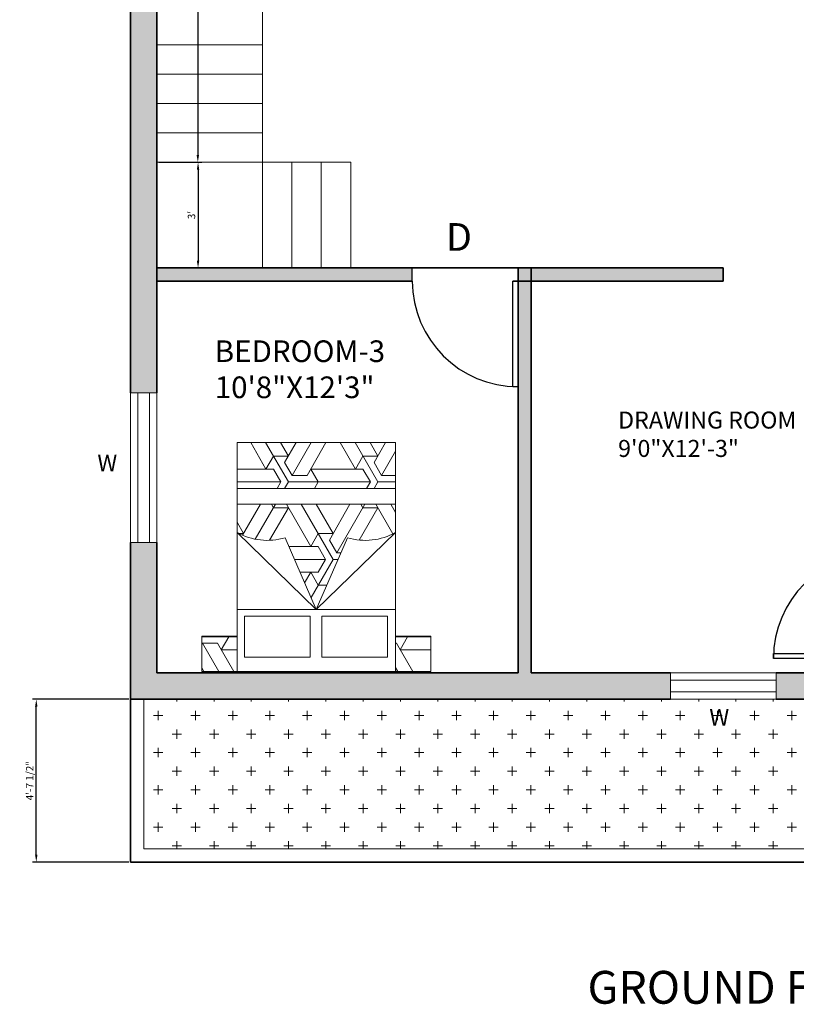
# Model space of a CAD drawing. Units: inches. Extents: x 1878 to 2382, y 1889 to 2524.
# Tile 1 of 2: x 1878 to 2143, y 1889 to 2225. Entities that reach past the tile are written whole.
import ezdxf

# ---------------------------------------------------------------- set-up
doc = ezdxf.new("R2010")
doc.units = ezdxf.units.IN
for name, color, linetype, lineweight in [('A-ANNO-DIMS', 2, 'Continuous', 18), ('A-ANNO-TEXT', 7, 'Continuous', 18), ('A-ANNO-TITL', 7, 'Continuous', 30), ('A-AREA-IDEN', 7, 'Continuous', 18), ('A-DOOR', 4, 'Continuous', 25), ('A-FLOR-STRS', 7, 'Continuous', 18), ('A-FURN', 8, 'Continuous', 18), ('A-FURN-PATT', 252, 'Continuous', 13), ('A-WALL', 7, 'Continuous', 35), ('A-WALL-PATT', 251, 'Continuous', 13), ('L-PLNT', 3, 'Continuous', 18), ('L-PLNT-PATT', 3, 'Continuous', 13), ('windows', 5, 'Continuous', 18)]:
    doc.layers.add(name, color=color, linetype=linetype, lineweight=lineweight)
doc.styles.get("Standard").update_dxf_attribs({"font": 'arial.ttf'})
doc.dimstyles.new('ISO-25', dxfattribs={"dimtxt": 2.5, "dimasz": 2.5, "dimexe": 1.25, "dimexo": 0.625, "dimtad": 1, "dimlunit": 3, "dimtxsty": 'Standard', "dimcen": 2.5, "dimadec": 0, "dimazin": 0, "dimtfac": 1, "dimtmove": 0, "dimatfit": 3, "dimfxl": 1, "dimarcsym": 0})

# ---------------------------------------------------------------- blocks, each defined once
blk = doc.blocks.new('*D9')
at = {"layer": 'A-ANNO-DIMS', "color": 0, "lineweight": -2, "transparency": 16777216}
for p, q in [((1925.866440692248, 2286.068149098085), (1940.420566168725, 2286.068149098085)), ((1939.170566168725, 2283.568149098085), (1939.170566168725, 2178.568149098085)), ((1925.866440692248, 2176.068149098085), (1940.420566168725, 2176.068149098085))]:
    blk.add_line(p, q, dxfattribs=at)
at = {"layer": 'A-ANNO-DIMS', "color": 0, "transparency": 16777216}
for points in [[(1938.753899502058, 2283.568149098085), (1939.587232835391, 2283.568149098085), (1939.170566168725, 2286.068149098085)], [(1938.753899502058, 2178.568149098085), (1939.587232835391, 2178.568149098085), (1939.170566168725, 2176.068149098085)]]:
    blk.add_solid(points, dxfattribs=at)
at = {"layer": 'Defpoints', "color": 0, "transparency": 16777216}
for p in [(1925.241440692248, 2286.068149098085), (1925.241440692248, 2176.068149098085), (1939.170566168725, 2176.068149098085)]:
    blk.add_point(p, dxfattribs=at)
at = {"layer": 'A-ANNO-DIMS', "color": 0, "transparency": 16777216, "insert": (1937.269133699421, 2231.068149098084), "char_height": 2.5, "attachment_point": 5, "rotation": 90}
blk.add_mtext('9\'-2"', dxfattribs=at)
blk = doc.blocks.new('*D11')
at = {"layer": 'A-ANNO-DIMS', "color": 0, "lineweight": -2, "transparency": 16777216}
for p, q in [((1925.866440692248, 2176.068149098085), (1940.498560281259, 2176.068149098085)), ((1939.248560281259, 2173.568149098085), (1939.248560281259, 2142.568149098085)), ((1925.866440692248, 2140.068149098085), (1940.498560281259, 2140.068149098085))]:
    blk.add_line(p, q, dxfattribs=at)
at = {"layer": 'A-ANNO-DIMS', "color": 0, "transparency": 16777216}
for points in [[(1938.831893614593, 2173.568149098085), (1939.665226947926, 2173.568149098085), (1939.248560281259, 2176.068149098085)], [(1938.831893614593, 2142.568149098085), (1939.665226947926, 2142.568149098085), (1939.248560281259, 2140.068149098085)]]:
    blk.add_solid(points, dxfattribs=at)
at = {"layer": 'Defpoints', "color": 0, "transparency": 16777216}
for p in [(1925.241440692248, 2176.068149098085), (1925.241440692248, 2140.068149098085), (1939.248560281259, 2140.068149098085)]:
    blk.add_point(p, dxfattribs=at)
at = {"layer": 'A-ANNO-DIMS', "color": 0, "transparency": 16777216, "insert": (1937.346275151655, 2158.068149098085), "char_height": 2.5, "attachment_point": 5, "rotation": 90}
blk.add_mtext("3'", dxfattribs=at)
blk = doc.blocks.new('*U12')
for p, q in [((-36, 4e-16), (-36, 4)), ((0, 0), (0, 3.999999999999999))]:
    blk.add_line(p, q)
blk.add_lwpolyline([(0, 0), (-7.1e-15, -36), (-1.750000000000007, -36), (-1.75, 4e-16)], close=True)
blk.add_arc((0, 0), 36, 180, 270)
blk = doc.blocks.new('*U2')
for p, q in [((0, 0), (-1e-16, -3.999999999999999)), ((36, -4e-16), (36, -3.999999999999999))]:
    blk.add_line(p, q)
blk.add_lwpolyline([(0, 0), (5.2e-15, 36), (1.750000000000006, 36), (1.749999999999998, -7e-16)], close=True)
blk.add_arc((0, 0), 36, 0, 90)
blk = doc.blocks.new('BED-DOUBLE-WITH-NIGHTSTANDS')
for p, q in [((39.00041612759128, 21.08000700798311), (12.00041612759128, 47.34561457886321)), ((39.00041612759128, 21.08000700798311), (66.00041612759127, 47.34561457886321)), ((39.00041612759128, 21.08000700798311), (28.35091833014235, 45.54110342781223)), ((39.00041612759128, 21.08000700798311), (49.64991392504021, 45.54110342781223)), ((66.00041612759127, 21.08000700798311), (12.00041612759128, 21.08000700798311)), ((36.91574546573361, 4.839445541926579), (36.91574546573361, 18.8744984206578)), ((40.91574546573361, 4.839445541926579), (40.91574546573361, 18.8744984206578)), ((0.0004161275912793, 0.0002775178572847), (0.0004161275912793, 12.00027751785728)), ((0.0004161275912793, 12.00027751785728), (12.00041612759128, 12.00027751785728)), ((78.00041612759128, 12.00027751785728), (66.00041612759127, 12.00027751785728)), ((78.00041612759128, 12.00027751785728), (78.00041612759128, 0.0002775178572847)), ((12.00041612759128, 0.0002775178572847), (0.0004161275912793, 0.0002775178572847)), ((66.00041612759127, 0.0002775178572847), (78.00041612759128, 0.0002775178572847))]:
    blk.add_line(p, q)
for points in [[(66.00041612759127, 78.00027751785728), (12.00041612759128, 78.00027751785728), (12.00041612759128, 0.0002775178572847), (66.00041612759127, 0.0002775178572847)], [(66.00041612759127, 56.96965028294471), (12.00041612759128, 56.96965028294471), (12.00041612759128, 62.38317077163083), (66.00041612759127, 62.38317077163083)]]:
    blk.add_lwpolyline(points, close=True)
for points in [[(36.91574546573361, 4.839445541926579), (14.53815381501522, 4.839445541926579), (14.53815381501522, 18.8744984206578), (36.91574546573361, 18.8744984206578)], [(40.91574546573361, 18.8744984206578), (63.29333711645199, 18.8744984206578), (63.29333711645199, 4.839445541926579), (40.91574546573361, 4.839445541926579)]]:
    blk.add_lwpolyline(points)
for centre, start, end in [((22.35293988504668, 66.17141739726458), 241.1931034301566, 286.2110586149389), ((55.64789237013588, 66.17141739726458), 253.7889413850611, 298.8068965698434)]:
    blk.add_arc(centre, 21.48454327897181, start, end)
blk = doc.blocks.new('WIN-51IN')
for p, q in [((4.500440692245319, 51.00020935019097), (0.0004406922455473, 51.00020935019074)), ((0.0004406922455473, 51.00020935019074), (9.000440692245093, 51.00020935019142)), ((0.0004406922482758, 0.0002093501907439), (0.0004406922441831, 51.00020935019074)), ((2.500440692248048, 0.0002093501907439), (2.500440692245319, 51.00020935019097)), ((6.500440692248048, 0.0002093501911986), (6.500440692245319, 51.0002093501912)), ((9.000440692245318, 51.0002093501912), (9.000440692247594, 0.0002093501911986)), ((0.0004406922482758, 0.0002093501907439), (9.000440692247821, 0.0002093501911986)), ((9.000440692247821, 0.0002093501911986), (4.500440692248048, 0.0002093501911986))]:
    blk.add_line(p, q)
blk = doc.blocks.new('*D27')
at = {"layer": 'A-ANNO-DIMS', "color": 0, "lineweight": -2, "transparency": 16777216}
for p, q in [((1915.616441000001, 1993.068149000001), (1882.891441000001, 1993.068149000001)), ((1884.141441000002, 1940.068149000001), (1884.141441000002, 1990.568149000001)), ((1915.616441000001, 1937.568149000001), (1882.891441000001, 1937.568149000001))]:
    blk.add_line(p, q, dxfattribs=at)
at = {"layer": 'A-ANNO-DIMS', "color": 0, "transparency": 16777216}
for points in [[(1883.724774333335, 1990.568149000001), (1884.558107666668, 1990.568149000001), (1884.141441000002, 1993.068149000001)], [(1883.724774333335, 1940.068149000001), (1884.558107666668, 1940.068149000001), (1884.141441000002, 1937.568149000001)]]:
    blk.add_solid(points, dxfattribs=at)
at = {"layer": 'Defpoints', "color": 0, "transparency": 16777216}
for p in [(1884.141441000002, 1993.068149000001), (1916.241441000001, 1993.068149000001), (1916.241441000001, 1937.568149000001)]:
    blk.add_point(p, dxfattribs=at)
at = {"layer": 'A-ANNO-DIMS', "color": 0, "transparency": 16777216, "insert": (1882.223807984995, 1965.318148999999), "char_height": 2.5, "attachment_point": 5, "rotation": 90}
blk.add_mtext('4\'-7 1/2"', dxfattribs=at)

msp = doc.modelspace()

# ---------------------------------------------------------------- hatches: boundary and pattern name
at = {"layer": 'A-FURN-PATT'}
h = msp.add_hatch(dxfattribs=at)
h.set_pattern_fill('ESCHER', color=256, angle=180)
h.set_pattern_definition([(240, (4377.911806630984, 4495.575865926148), (30.47999998809242, 6.8748365e-09), [27.94, -2.539999999999999]), (360, (4377.911806630984, 4495.575865926148), (-15.23999999999999, 26.39645429360001), [27.94, -2.54]), (120, (4377.911806630984, 4495.575865926148), (-30.47999998809242, 6.874844e-09), [27.94, -2.539999999999999]), (240, (4375.371806630983, 4495.575865926148), (30.47999998809242, 6.8748365e-09), [5.079999999999999, -25.4]), (120, (4375.371806630983, 4495.575865926148), (-30.47999998809242, 6.874844e-09), [5.079999999999999, -25.4]), (240, (4379.181806630984, 4493.376161410148), (30.47999998809242, 6.8748365e-09), [5.079999999999999, -25.4]), (360, (4379.181806630984, 4493.376161410148), (-15.23999999999999, 26.39645429360001), [5.08, -25.4]), (120, (4379.181806630984, 4497.775570442148), (-30.47999998809242, 6.874844e-09), [5.079999999999999, -25.4]), (360, (4379.181806630984, 4497.775570442148), (-15.23999999999999, 26.39645429360001), [5.08, -25.4]), (240, (4388.071806630984, 4495.575865926148), (30.47999998809242, 6.8748365e-09), [5.079999999999999, -25.4]), (120, (4388.071806630984, 4495.575865926148), (-30.47999998809242, 6.874844e-09), [5.079999999999999, -25.4]), (240, (4372.831806630983, 4504.374684015548), (30.47999998809242, 6.8748365e-09), [5.079999999999999, -25.4]), (360, (4372.831806630983, 4504.374684015548), (-15.23999999999999, 26.39645429360001), [5.08, -25.4]), (120, (4372.831806630983, 4486.777047836748), (-30.47999998809242, 6.874844e-09), [5.079999999999999, -25.4]), (360, (4372.831806630983, 4486.777047836748), (-15.23999999999999, 26.39645429360001), [5.08, -25.4]), (180, (4372.831806630983, 4491.176456868749), (15.24, -26.39645429360001), [17.78, -12.7]), (180, (4372.831806630983, 4499.975274983547), (15.24, -26.39645429360001), [17.78, -12.7]), (300, (4376.641806630983, 4488.976752352748), (30.47999998809242, -6.8748546e-09), [17.78, -12.7]), (300, (4384.261806630984, 4493.376161410148), (30.47999998809242, -6.8748546e-09), [17.78, -12.7]), (59.99999999999997, (4384.261806630984, 4497.775570442148), (-15.2399999880924, 26.39645430047486), [17.78, -12.7]), (59.99999999999997, (4376.641806630983, 4502.174979499549), (-15.2399999880924, 26.39645430047486), [17.78, -12.7])])
h.paths.add_polyline_path([(1979.526416127591, 2023.596007007983), (1990.17591392504, 2048.057103427812, 0.1989938127017903), (2006.526416127591, 2049.861614578864), (2006.526416127591, 2059.485650282945), (1952.526416127591, 2059.485650282945), (1952.526416127591, 2049.861614578863, 0.1989938127017848), (1968.876918330142, 2048.057103427812)])
h.paths.add_polyline_path([(1952.526416127591, 2064.899170771631), (2006.526416127591, 2064.899170771631), (2006.526416127591, 2080.516277517857), (1952.526416127591, 2080.516277517857)])
h.paths.add_polyline_path([(1940.526416127591, 2002.516277517857), (1952.526416127591, 2002.516277517857), (1952.526416127591, 2014.516277517858), (1940.526416127591, 2014.516277517858)])
h.paths.add_polyline_path([(2006.526416127591, 2002.516277517857), (2018.526416127591, 2002.516277517857), (2018.526416127591, 2014.516277517858), (2006.526416127591, 2014.516277517858)])
at = {"layer": 'A-WALL-PATT'}
h = msp.add_hatch(color=256, dxfattribs=at)
h.dxf.hatch_style = 1
h.paths.add_polyline_path([(1925.241440692247, 2376.261341107433), (1916.241440692247, 2376.261341107433), (1916.241440692247, 2322.068149098084), (1920.741440692247, 2322.068149098084), (1925.241440692247, 2322.068149098084)])
h.paths.add_polyline_path([(1925.241440692247, 2286.140121582637), (1916.241440692247, 2286.068149098084), (1916.241440692247, 2097.50720935019), (1920.741440692247, 2097.50720935019), (1925.241440692246, 2097.50720935019)])
h.paths.add_polyline_path([(1925.241440692246, 2046.50720935019), (1916.241440692247, 2046.50720935019), (1916.241440692247, 1993.068149098084), (1925.241440692247, 1993.068149098084), (2100.228537208572, 1993.068149098084), (2100.228537208572, 1997.568149098084), (2100.228537208572, 2002.068149098084), (2052.741440692247, 2002.068149098084), (2052.741440692247, 2135.568149098084), (2048.241440692248, 2135.568149098084), (2048.241440692248, 2002.068149098084), (1925.241440692246, 2002.068149098084)])
h.paths.add_polyline_path([(2175.741440692247, 2006.934770096195), (2175.253494205439, 2006.934770096195), (2171.241440692247, 2006.934770096195), (2171.241440692247, 2002.068149098084), (2136.228537208572, 2002.068149098084), (2136.228537208572, 1993.068149098084), (2171.241440692247, 1993.068149098084), (2175.741440692247, 1993.068149098084)])
h.paths.add_polyline_path([(1925.241440692247, 2492.568149098084), (2018.709393843749, 2492.568149098085), (2018.709393843749, 2497.068149098084), (2018.709393843749, 2501.568149098084), (1916.241440692247, 2501.568149098084), (1916.241440692247, 2427.261341107433), (1925.241440692247, 2427.261341107433)])
h.paths.add_polyline_path([(2324.241440692247, 2501.568149098084), (2052.741440692247, 2501.568149098084), (2052.741440692247, 2497.068149098084), (2319.741440692247, 2497.068149098084), (2319.741440692247, 2446.568149098084), (2324.241440692247, 2446.568149098084)])
h.paths.add_polyline_path([(2110.637963685758, 2446.568149098085), (2052.741440692248, 2446.568149098085), (2052.741440692247, 2492.568149098085), (2048.241440692248, 2492.568149098085), (2048.241440692248, 2446.568149098084), (1976.241440692247, 2446.568149098084), (1976.241440692247, 2442.068149098084), (2048.241440692248, 2442.068149098084), (2048.241440692248, 2326.568149098084), (2052.741440692248, 2326.568149098084), (2052.741440692248, 2442.068149098085), (2110.637963685758, 2442.068149098085), (2110.637963685758, 2444.318149098084)])
h.paths.add_polyline_path([(2100.741440692248, 2326.568149098084), (2052.741440692248, 2326.568149098084), (2052.741440692248, 2322.068149098084), (2100.741440692248, 2322.068149098084)])
h.paths.add_polyline_path([(2052.741440692248, 2326.568149098084), (2048.241440692248, 2326.568149098084), (2048.241440692248, 2322.068149098084), (2052.741440692248, 2322.068149098084)])
h.paths.add_polyline_path([(2048.241440692248, 2326.568149098084), (2045.469072311536, 2326.568149098084), (2045.469072311536, 2326.564566759995), (2045.469072311536, 2322.564566759995), (2045.469072311536, 2322.068149098084), (2048.241440692248, 2322.068149098084)])
h.paths.add_polyline_path([(2009.469072311536, 2326.568149098084), (1925.241440692247, 2326.568149098084), (1925.241440692247, 2322.068149098084), (2009.469072311536, 2322.068149098084), (2009.469072311536, 2322.564566759995)])
h.paths.add_polyline_path([(2315.241440692247, 2326.568149098084), (2259.241440692248, 2326.568149098084), (2259.241440692247, 2405.455505715361), (2255.232373025363, 2405.455505715361), (2254.741440692247, 2405.455505715361), (2254.741440692247, 2326.568149098084), (2207.241440692247, 2326.568149098084), (2195.241440692247, 2326.568149098084), (2195.241440692247, 2322.068149098084), (2207.241440692247, 2322.068149098084), (2207.241440692247, 2317.983016143046), (2207.736123013865, 2317.983016143046), (2211.741440692247, 2317.983016143046), (2211.741440692247, 2322.068149098084), (2315.241440692247, 2322.068149098084)])
h.paths.add_polyline_path([(2315.241440692247, 2446.568149098084), (2161.637963685759, 2446.568149098084), (2161.637963685759, 2442.068149098084), (2254.741440692248, 2442.068149098084), (2254.741440692248, 2435.45550571536), (2255.232373025363, 2435.45550571536), (2259.241440692247, 2435.45550571536), (2259.241440692247, 2442.068149098084), (2315.241440692247, 2442.068149098084)])
h.paths.add_polyline_path([(2315.241440692247, 2274.068149098084), (2207.241440692247, 2274.068149098084), (2171.241440692247, 2274.068149098084), (2171.241440692247, 2265.326277142973), (2171.730927479741, 2265.326277142973), (2175.741440692247, 2265.326277142973), (2175.741440692247, 2269.568149098084), (2315.241440692247, 2269.568149098084)])
h.paths.add_polyline_path([(2226.77806988673, 2011.848788610063), (2261.830806516837, 2011.848788610063), (2261.830806516837, 2029.016856799895), (2226.77806988673, 2029.016856799895)], flags=9)
h.paths.add_polyline_path([(2187.32039703604, 2282.173908487125), (2191.179537554457, 2282.173908487125), (2191.179537554457, 2287.32568202055), (2187.32039703604, 2287.32568202055)], flags=9)
h.paths.add_polyline_path([(2140.303776002406, 2010.813127097478), (2177.357239682197, 2010.813127097478), (2177.357239682197, 2025.39985028964), (2140.303776002406, 2025.39985028964)], flags=9)
h.paths.add_polyline_path([(2106.34299009357, 2361.376149589321), (2203.937232242951, 2361.376149589321), (2203.937232242951, 2388.800664716006), (2106.34299009357, 2388.800664716006)], flags=9)
h.paths.add_polyline_path([(2229.025427119923, 2239.685701226347), (2287.845526911306, 2239.685701226347), (2287.845526911306, 2264.045270653161), (2229.025427119923, 2264.045270653161)], flags=9)
h.paths.add_polyline_path([(2039.469638618838, 2246.05759564136), (2106.461015502027, 2246.05759564136), (2106.461015502027, 2270.434976204787), (2039.469638618838, 2270.434976204787)], flags=9)
h.paths.add_polyline_path([(2080.263524544797, 2072.342763218177), (2149.799479349807, 2072.342763218177), (2149.799479349807, 2093.991209603414), (2080.263524544797, 2093.991209603414)], flags=9)
h = msp.add_hatch(color=256, dxfattribs=at)
h.dxf.hatch_style = 1
h.paths.add_polyline_path([(2118.158477370382, 2140.068149098084), (2052.741440692247, 2140.068149098084), (2052.741440692247, 2135.568149098084), (2118.158477370382, 2135.568149098084)])
h.paths.add_polyline_path([(2012.241440692247, 2139.568149098084), (2012.241440692247, 2140.068149098084), (1925.241440692246, 2140.068149098084), (1925.241440692246, 2135.568149098084), (2012.241440692247, 2135.568149098084)])
h.paths.add_polyline_path([(2052.741440692247, 2140.068149098084), (2048.241440692248, 2140.068149098084), (2048.241440692248, 2135.568149098084), (2052.741440692247, 2135.568149098084)])
at = {"layer": 'L-PLNT-PATT'}
h = msp.add_hatch(dxfattribs=at)
h.set_pattern_fill('CROSS', color=256)
h.set_pattern_definition([(0, (0, 0), (6.349999999999999, 6.349999999999999), [3.174999999999999, -9.525]), (90, (1.587499999999999, -1.587499999999999), (-6.349999999999999, 6.349999999999999), [3.174999999999999, -9.525])])
h.paths.add_polyline_path([(2175.741440692247, 1942.068149098084), (2175.741440692247, 1993.068149098084), (2171.241440692247, 1993.068149098084), (2136.228537208572, 1993.068149098084), (2100.228537208572, 1993.068149098084), (1925.241440692247, 1993.068149098084), (1920.741440692247, 1993.068149098084), (1920.741440692247, 1942.068149098084)])

# ---------------------------------------------------------------- linework, layer by layer
at = {"layer": 'A-DOOR'}
msp.add_line((2012.241440692247, 2139.568149098084), (2012.241440692247, 2140.068149098084), dxfattribs=at)
at = {"layer": 'A-FLOR-STRS'}
for p, q in [((1925.241440692247, 2286.068149098084), (1925.241440692247, 2176.068149098084)), ((1961.241440692247, 2276.068149098084), (1961.241440692247, 2176.068149098084)), ((1961.241440692247, 2216.068149098084), (1925.241440692247, 2216.068149098084)), ((1961.241440692247, 2206.068149098084), (1925.241440692247, 2206.068149098084)), ((1961.241440692247, 2196.068149098084), (1925.241440692247, 2196.068149098084)), ((1961.241440692247, 2186.068149098084), (1925.241440692247, 2186.068149098084)), ((1925.241440692247, 2176.068149098084), (1961.241440692247, 2176.068149098084)), ((1925.241440692247, 2176.068149098084), (1925.241440692247, 2140.068149098084)), ((1961.241440692247, 2176.068149098084), (1961.241440692247, 2140.068149098084)), ((1961.241440692247, 2176.068149098084), (1991.241440692247, 2176.068149098084)), ((1971.241440692247, 2176.068149098084), (1971.241440692247, 2140.068149098084)), ((1981.241440692247, 2176.068149098084), (1981.241440692247, 2140.068149098084)), ((1991.241440692247, 2176.068149098084), (1991.241440692247, 2140.068149098084))]:
    msp.add_line(p, q, dxfattribs=at)
at = {"layer": 'A-WALL'}
for p, q in [((1916.241440692247, 2097.50720935019), (1916.241440692247, 2286.068149098084)), ((1925.241440692246, 2097.50720935019), (1925.241440692247, 2286.140121582637)), ((1925.241440692247, 2140.068149098084), (2052.741440692248, 2140.068149098084)), ((2048.241440692248, 2002.068149098084), (2048.241440692248, 2140.068149098085)), ((2052.741440692247, 2002.068149098084), (2052.741440692247, 2140.068149098084)), ((2052.741440692248, 2140.068149098084), (2118.158477370382, 2140.068149098084)), ((2118.158477370382, 2140.068149098084), (2118.158477370382, 2135.568149098084)), ((1925.241440692247, 2135.568149098084), (2012.241440692247, 2135.568149098084)), ((2046.491440692247, 2135.568149098084), (2052.741440692248, 2135.568149098084)), ((2052.741440692248, 2135.568149098084), (2118.158477370382, 2135.568149098084)), ((1916.241440692247, 1937.568149098084), (1916.241440692247, 2046.50720935019)), ((1925.241440692246, 2002.068149098084), (1925.241440692246, 2046.507209350191)), ((2048.241440692248, 2002.068149098084), (1925.241440692247, 2002.068149098084)), ((2100.228537208572, 2002.068149098084), (2052.741440692247, 2002.068149098084)), ((2171.241440692247, 2002.068149098084), (2136.228537208572, 2002.068149098084)), ((1925.241440692247, 1993.068149098084), (1916.241440692247, 1993.068149098084)), ((2100.228537208572, 1993.068149098084), (1925.241440692247, 1993.068149098084)), ((2171.241440692247, 1993.068149098084), (2136.228537208572, 1993.068149098084)), ((2175.741440692247, 1937.568149098084), (1916.241440692247, 1937.568149098084))]:
    msp.add_line(p, q, dxfattribs=at)
at = {"layer": 'L-PLNT'}
for q in [(1920.741440692246, 1993.068149098084), (2175.74144069224, 1942.068149098084)]:
    msp.add_line((1920.741440692247, 1942.068149098084), q, dxfattribs=at)
at = {"layer": 'windows'}
for p, q in [((2100.228537208572, 2002.068149098084), (2100.228537208572, 1993.068149098084)), ((2136.228537208572, 2002.068149098084), (2100.228537208572, 2002.068149098084)), ((2136.228537208572, 1997.568149098084), (2136.228537208572, 2002.068149098084)), ((2136.228537208572, 2002.068149098084), (2136.228537208572, 1993.068149098084)), ((2100.228537208572, 1999.568149098084), (2136.228537208572, 1999.568149098084)), ((2100.228537208572, 1993.068149098084), (2100.228537208572, 1997.568149098084)), ((2100.228537208572, 1995.568149098084), (2136.228537208572, 1995.568149098084)), ((2100.228537208572, 1993.068149098084), (2136.228537208572, 1993.068149098084))]:
    msp.add_line(p, q, dxfattribs=at)

# ---------------------------------------------------------------- block references
at = {"layer": 'A-DOOR'}
msp.add_blockref('*U12', (2048.241440692248, 2135.568149098084), dxfattribs=at)
at = {"layer": 'A-DOOR', "rotation": 90}
msp.add_blockref('*U2', (2171.253494205439, 2006.934770096195), dxfattribs=at)
at = {"layer": 'A-FURN'}
msp.add_blockref('BED-DOUBLE-WITH-NIGHTSTANDS', (1940.526, 2002.516), dxfattribs=at)
at = {"layer": 'windows', "rotation": 180}
msp.add_blockref('WIN-51IN', (1925.241881384495, 2097.507418700381), dxfattribs=at)

# ---------------------------------------------------------------- texts
at = {"layer": 'A-ANNO-TEXT', "attachment_point": 1}
for s, width, gutter_width, insert, char_height in [('D', 211.869678819047, 47.15432065229713, (2023.693826606333, 2155.329521521891), 9.430864130459426), ('W', 334.9241299264371, 28.12125752358024, (1904.967440970025, 2076.407930946428), 5.624251504716047), ('W', 334.9241299264371, 28.12125752358024, (2113.422631469629, 1989.678805785211), 5.624251504716047)]:
    msp.add_mtext_dynamic_manual_height_columns(s, width=width, gutter_width=gutter_width, heights=[0], dxfattribs=dict(at, insert=insert, char_height=char_height))
at = {"layer": 'A-ANNO-TITL', "insert": (2071.913172093511, 1900.47408762042), "char_height": 11.1892339464713, "attachment_point": 1}
msp.add_mtext_dynamic_manual_height_columns('GROUND FLOOR PLAN', width=187.0432349417984, gutter_width=55.9461697323565, heights=[0], dxfattribs=at)
at = {"layer": 'A-AREA-IDEN', "attachment_point": 1}
for s, width, gutter_width, insert, char_height in [('BEDROOM-3\\P10\'8"X12\'3"', 81.64539776399761, 36.8856547814649, (1944.933796447963, 2115.354813693245), 7.37713095629298), ('DRAWING ROOM\\P9\'0"X12\'-3"\\P\\P  ', 106.0798166384483, 29.00794199082112, (2082.339195155191, 2091.108223827109), 5.801588398164224)]:
    msp.add_mtext_dynamic_manual_height_columns(s, width=width, gutter_width=gutter_width, heights=[0], dxfattribs=dict(at, insert=insert, char_height=char_height))

# ---------------------------------------------------------------- dimensions: what is measured, and where the dimension line sits
at = {"layer": 'A-ANNO-DIMS'}
for base, p1, p2, override, picture, middle in [((1939.170566168725, 2176.068149098085), (1925.241440692247, 2286.068149098084), (1925.241440692247, 2176.068149098084), {"dimclrd": 0, "dimclre": 0, "dimclrt": 0}, '*D9', (1937.269133699421, 2231.068149098084)), ((1939.248560281259, 2140.068149098085), (1925.241440692247, 2176.068149098084), (1925.241440692247, 2140.068149098084), {"dimclrd": 0, "dimclre": 0, "dimclrt": 0}, '*D11', (1937.346275151655, 2158.068149098085)), ((1884.141441000002, 1993.068149000001), (1916.241441, 1937.568149), (1916.241441, 1993.068149), {"dimdec": 1, "dimlfac": 1, "dimrnd": 0, "dimzin": 1, "dimdsep": 46, "dimlunit": 4, "dimfrac": 2}, '*D27', (1882.223807984995, 1965.318148999999))]:
    dim = msp.add_linear_dim(base=base, p1=p1, p2=p2, angle=90, dimstyle='ISO-25', override=override, dxfattribs=at)
    dim.commit()
    dim.dimension.update_dxf_attribs({"geometry": picture, "text_midpoint": middle})

doc.saveas('drawing.dxf')
